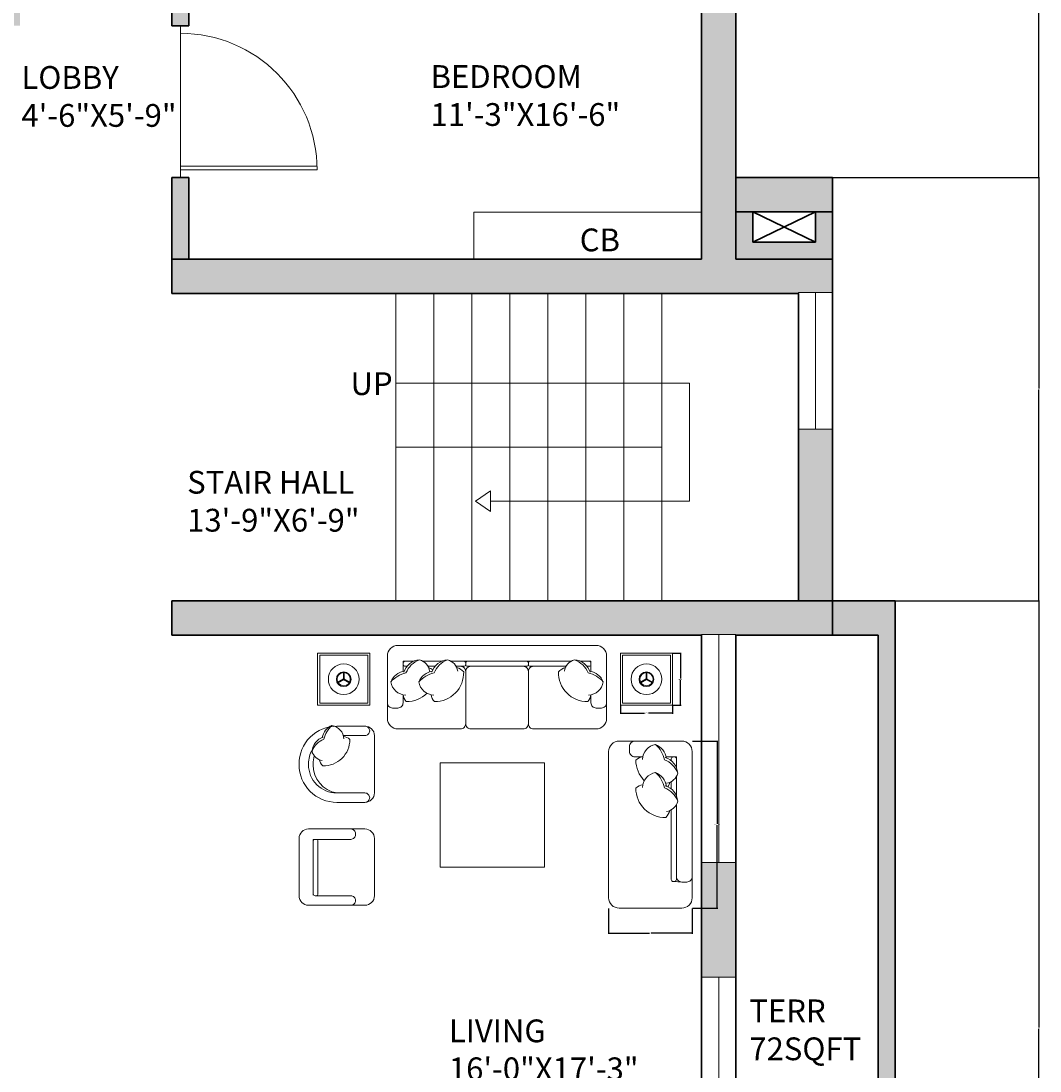
# Model space of a CAD drawing. Units: inches. Extents: x -36 to 442, y -676 to 151.
# Tile 4 of 8: x 174 to 442, y -411 to -134. Entities that reach past the tile are written whole.
import ezdxf

# ---------------------------------------------------------------- set-up
doc = ezdxf.new("R2010")
doc.units = ezdxf.units.IN
doc.header["$MEASUREMENT"] = 0
for name, color, linetype, lineweight in [('A-ANNO-DIMS', 2, 'Continuous', 18), ('A-ANNO-SYMB', 7, 'Continuous', 18), ('A-ANNO-TEXT', 7, 'Continuous', 18), ('A-AREA-IDEN', 7, 'Continuous', 18), ('A-DOOR', 4, 'Continuous', 18), ('A-FLOR-CASE', 32, 'Continuous', 18), ('A-FLOR-STRS', 7, 'Continuous', 18), ('A-FURN', 9, 'Continuous', 13), ('A-GLAZ', 4, 'Continuous', 13), ('A-WALL', 7, 'Continuous', 35), ('A-WALL-PATT', 8, 'Continuous', 13)]:
    doc.layers.add(name, color=color, linetype=linetype, lineweight=lineweight)
doc.styles.get("Standard").update_dxf_attribs({"font": 'arial.ttf'})
doc.dimstyles.get("Standard").update_dxf_attribs({"dimtxt": 0.18, "dimasz": 0.18, "dimexe": 0.18, "dimexo": 0.0625, "dimgap": 0.09, "dimtad": 0, "dimtih": 1, "dimtoh": 1, "dimdec": 0, "dimzin": 0, "dimdsep": 46, "dimlunit": 3, "dimtxsty": 'Standard', "dimcen": 0.09, "dimadec": 0, "dimazin": 0, "dimtfac": 1, "dimtdec": 0, "dimtofl": 0, "dimtmove": 0, "dimatfit": 3, "dimfxl": 1, "dimtolj": 1, "dimtzin": 0, "dimarcsym": 0})

# ---------------------------------------------------------------- blocks, each defined once
blk = doc.blocks.new('DAY BED1')
at = {"color": 0}
blk.add_line((0.3, 0.25), (0.225, 0.255), dxfattribs=at)
blk.add_lwpolyline([(-0.3, 0, -0.414214), (-0.4, 0.1), (-0.4, 0.1, 0.317837), (-0.4, 0.1, -0.414214), (-0.4, 0.1), (-0.4, 0.1, 1.186185), (-0.4, 0.1, -0.414214), (-0.4, 0.1), (-0.4, 1.5, -0.414214), (-0.3, 1.6), (0.3, 1.6, -0.414214), (0.4, 1.5), (0.4, 0.1, -0.414214), (0.3, 0)], format="xyb", close=True, dxfattribs=at)
for points in [[(-0.073, 1.45), (-0.15, 1.45, -0.414214), (-0.2, 1.5), (-0.2, 1.55, -0.414214), (-0.15, 1.6)], [(-0.076, 1.425, -0.356772), (0.05, 1.568, -0.249542), (0.154, 1.438, 9.61688)], [(0.05, 1.568, -0.14773), (0.136, 1.422, -0.213343), (0.262, 1.293, -0.178662)], [(-0.073, 1.45, 0.165541), (-0.139, 1.419, 0.200231), (-0.058, 1.221, 0.121523)], [(0.143, 1.442, -0.306663), (0.262, 1.293, -0.30633), (0.154, 1.196, 0.872847)], [(0.25, 1.345), (0.25, 1.45), (0.152, 1.45, -0.414214)], [(0.2, 1.412), (0.2, 1.43, -0.414214), (0.22, 1.45), (0.23, 1.45, -0.414214), (0.25, 1.43)], [(0.25, 1.43), (0.25, 1.345, -0.414214)], [(-0.076, 1.156, -0.356772), (0.05, 1.299, -0.249542), (0.154, 1.169, 9.61688)], [(0.05, 1.299, -0.14773), (0.136, 1.153, -0.213343), (0.262, 1.024, -0.178662)], [(0.2, 1.142), (0.2, 1.211, -0.414214)], [(0.25, 1.262), (0.25, 1.075, -0.414214)], [(-0.073, 1.181, 0.165541), (-0.139, 1.15, 0.425989), (0.148, 0.869, 0.121523), (0.187, 0.936, -7.115464)], [(0.143, 1.173, -0.306663), (0.262, 1.024, -0.30633), (0.154, 0.926, 0.872847)], [(0.168, 1.163, 0.071865), (0.187, 1.205, -7.115464)], [(0.25, 0.992), (0.25, 0.275, -0.414214), (0.23, 0.255), (0.22, 0.255, -0.414214), (0.2, 0.275), (0.2, 0.942, -0.414214)], [(0.25, 0.377), (0.25, 0.3, 0.414214), (0.3, 0.25), (0.35, 0.25, 0.414214), (0.4, 0.3)]]:
    blk.add_lwpolyline(points, format="xyb", dxfattribs=at)
for points in [[(0.25, 1.075), (0.25, 1.262)], [(0.25, 0.377), (0.25, 0.992)]]:
    blk.add_lwpolyline(points, dxfattribs=at)
blk = doc.blocks.new('END-TABLE-SQUARE')
for p, q in [((6.79, 6.87), (6.79, 8.81)), ((6.96, 6.87), (6.96, 8.81)), ((6.83, 6.95), (5.15, 5.98)), ((6.92, 6.8), (5.24, 5.83)), ((6.83, 6.8), (8.51, 5.83)), ((6.92, 6.95), (8.59, 5.98))]:
    blk.add_line(p, q)
at = {"ltscale": 0.03}
blk.add_lwpolyline([(13.75, 0), (0, 0), (0, 13.75), (13.75, 13.75)], close=True, dxfattribs=at)
blk.add_lwpolyline([(0.55, 0.55), (13.2, 0.55), (13.2, 13.2), (0.55, 13.2)], close=True)
for radius in [4.05, 1.94, 1.74]:
    blk.add_circle((6.87, 6.87), radius)
blk = doc.blocks.new('GLAZING-UNIT-96IN')
for p, q in [((0, 0), (0, 96)), ((4.5, 96), (4.5, 0)), ((9, 96), (9, 0))]:
    blk.add_line(p, q)
blk = doc.blocks.new('*D37')
at = {"layer": 'A-ANNO-DIMS', "color": 0, "lineweight": -2, "transparency": 16777216}
for p, q in [((350.8, -323.93), (357.52, -323.93)), ((357.34, -324.11), (357.34, -345.74)), ((357.34, -367.74), (357.34, -346.1)), ((350.8, -367.92), (357.52, -367.92))]:
    blk.add_line(p, q, dxfattribs=at)
at = {"layer": 'A-ANNO-DIMS', "color": 0, "transparency": 16777216}
for points in [[(357.31, -324.11), (357.37, -324.11), (357.34, -323.93)], [(357.31, -367.74), (357.37, -367.74), (357.34, -367.92)]]:
    blk.add_solid(points, dxfattribs=at)
at = {"layer": 'Defpoints', "color": 0, "transparency": 16777216}
for p in [(350.74, -323.93), (357.34, -323.93), (350.74, -367.92)]:
    blk.add_point(p, dxfattribs=at)
at = {"layer": 'A-ANNO-DIMS', "color": 0, "transparency": 16777216, "insert": (357.34, -345.92), "char_height": 0.18, "attachment_point": 5}
blk.add_mtext('\\A1;DAY BED 44', dxfattribs=at)
blk = doc.blocks.new('*D38')
at = {"layer": 'A-ANNO-DIMS', "color": 0, "lineweight": -2, "transparency": 16777216}
for p, q in [((328.75, -367.98), (328.75, -374.69)), ((350.74, -367.98), (350.74, -374.69)), ((328.93, -374.51), (339.53, -374.51)), ((350.56, -374.51), (339.96, -374.51))]:
    blk.add_line(p, q, dxfattribs=at)
at = {"layer": 'A-ANNO-DIMS', "color": 0, "transparency": 16777216}
for points in [[(328.93, -374.48), (328.93, -374.54), (328.75, -374.51)], [(350.56, -374.48), (350.56, -374.54), (350.74, -374.51)]]:
    blk.add_solid(points, dxfattribs=at)
at = {"layer": 'Defpoints', "color": 0, "transparency": 16777216}
for p in [(328.75, -367.92), (350.74, -367.92), (350.74, -374.51)]:
    blk.add_point(p, dxfattribs=at)
at = {"layer": 'A-ANNO-DIMS', "color": 0, "transparency": 16777216, "insert": (339.74, -374.51), "char_height": 0.18, "attachment_point": 5}
blk.add_mtext('\\A1;22', dxfattribs=at)
blk = doc.blocks.new('*D39')
at = {"layer": 'A-ANNO-DIMS', "color": 0, "lineweight": -2, "transparency": 16777216}
for p, q in [((345.65, -300.75), (347.83, -300.75)), ((347.65, -300.93), (347.65, -307.44)), ((347.65, -314.31), (347.65, -307.8)), ((345.65, -314.49), (347.83, -314.49))]:
    blk.add_line(p, q, dxfattribs=at)
at = {"layer": 'A-ANNO-DIMS', "color": 0, "transparency": 16777216}
for points in [[(347.62, -300.93), (347.68, -300.93), (347.65, -300.75)], [(347.62, -314.31), (347.68, -314.31), (347.65, -314.49)]]:
    blk.add_solid(points, dxfattribs=at)
at = {"layer": 'Defpoints', "color": 0, "transparency": 16777216}
for p in [(345.58, -300.75), (347.65, -300.75), (345.58, -314.49)]:
    blk.add_point(p, dxfattribs=at)
at = {"layer": 'A-ANNO-DIMS', "color": 0, "transparency": 16777216, "insert": (347.65, -307.62), "char_height": 0.18, "attachment_point": 5}
blk.add_mtext('\\A1;TABLE 14 TYP.', dxfattribs=at)
blk = doc.blocks.new('*D40')
at = {"layer": 'A-ANNO-DIMS', "color": 0, "lineweight": -2, "transparency": 16777216}
for p, q in [((331.84, -314.56), (331.84, -316.74)), ((345.58, -314.56), (345.58, -316.74)), ((332.02, -316.56), (338.19, -316.56)), ((345.4, -316.56), (339.23, -316.56))]:
    blk.add_line(p, q, dxfattribs=at)
at = {"layer": 'A-ANNO-DIMS', "color": 0, "transparency": 16777216}
for points in [[(332.02, -316.53), (332.02, -316.59), (331.84, -316.56)], [(345.4, -316.53), (345.4, -316.59), (345.58, -316.56)]]:
    blk.add_solid(points, dxfattribs=at)
at = {"layer": 'Defpoints', "color": 0, "transparency": 16777216}
for p in [(331.84, -314.49), (345.58, -314.49), (345.58, -316.56)]:
    blk.add_point(p, dxfattribs=at)
at = {"layer": 'A-ANNO-DIMS', "color": 0, "transparency": 16777216, "insert": (338.71, -316.56), "char_height": 0.18, "attachment_point": 5}
blk.add_mtext('\\A1;14 TYP.', dxfattribs=at)
blk = doc.blocks.new('*D49')
at = {"layer": 'A-ANNO-DIMS', "color": 0, "lineweight": -2, "transparency": 16777216}
for p, q in [((2.24, -363.56), (2.24, -675.98)), ((404.24, -512.06), (404.24, -675.98)), ((2.42, -675.8), (202.94, -675.8)), ((404.06, -675.8), (203.53, -675.8))]:
    blk.add_line(p, q, dxfattribs=at)
at = {"layer": 'A-ANNO-DIMS', "color": 0, "transparency": 16777216}
for points in [[(2.42, -675.77), (2.42, -675.83), (2.24, -675.8)], [(404.06, -675.77), (404.06, -675.83), (404.24, -675.8)]]:
    blk.add_solid(points, dxfattribs=at)
at = {"layer": 'Defpoints', "color": 0, "transparency": 16777216}
for p in [(2.24, -363.5), (404.24, -512), (404.24, -675.8)]:
    blk.add_point(p, dxfattribs=at)
at = {"layer": 'A-ANNO-DIMS', "color": 0, "transparency": 16777216, "insert": (203.24, -675.8), "char_height": 0.18, "attachment_point": 5}
blk.add_mtext('\\A1;402', dxfattribs=at)
blk = doc.blocks.new('*D57')
at = {"layer": 'A-ANNO-DIMS', "color": 0, "lineweight": -2, "transparency": 16777216}
for p, q in [((378.8, 1), (442.22, 1)), ((442.04, 0.82), (442.04, -87.07)), ((442.04, -175.32), (442.04, -87.43)), ((387.8, -175.5), (442.22, -175.5))]:
    blk.add_line(p, q, dxfattribs=at)
at = {"layer": 'A-ANNO-DIMS', "color": 0, "transparency": 16777216}
for points in [[(442.01, 0.82), (442.07, 0.82), (442.04, 1)], [(442.01, -175.32), (442.07, -175.32), (442.04, -175.5)]]:
    blk.add_solid(points, dxfattribs=at)
at = {"layer": 'Defpoints', "color": 0, "transparency": 16777216}
for p in [(378.74, 1), (387.74, -175.5), (442.04, -175.5)]:
    blk.add_point(p, dxfattribs=at)
at = {"layer": 'A-ANNO-DIMS', "color": 0, "transparency": 16777216, "insert": (442.04, -87.25), "char_height": 0.18, "attachment_point": 5}
blk.add_mtext('\\A1;176.5', dxfattribs=at)
blk = doc.blocks.new('*D58')
at = {"layer": 'A-ANNO-DIMS', "color": 0, "lineweight": -2, "transparency": 16777216}
for p, q in [((387.8, -175.5), (442.22, -175.5)), ((442.04, -175.68), (442.04, -231.07)), ((442.04, -286.82), (442.04, -231.43)), ((404.3, -287), (442.22, -287))]:
    blk.add_line(p, q, dxfattribs=at)
at = {"layer": 'A-ANNO-DIMS', "color": 0, "transparency": 16777216}
for points in [[(442.01, -175.68), (442.07, -175.68), (442.04, -175.5)], [(442.01, -286.82), (442.07, -286.82), (442.04, -287)]]:
    blk.add_solid(points, dxfattribs=at)
at = {"layer": 'Defpoints', "color": 0, "transparency": 16777216}
for p in [(387.74, -175.5), (404.24, -287), (442.04, -287)]:
    blk.add_point(p, dxfattribs=at)
at = {"layer": 'A-ANNO-DIMS', "color": 0, "transparency": 16777216, "insert": (442.04, -231.25), "char_height": 0.18, "attachment_point": 5}
blk.add_mtext('\\A1;111.5', dxfattribs=at)
blk = doc.blocks.new('*D59')
at = {"layer": 'A-ANNO-DIMS', "color": 0, "lineweight": -2, "transparency": 16777216}
for p, q in [((404.3, -287), (442.22, -287)), ((442.04, -287.18), (442.04, -399.32)), ((442.04, -511.82), (442.04, -399.68)), ((404.3, -512), (442.22, -512))]:
    blk.add_line(p, q, dxfattribs=at)
at = {"layer": 'A-ANNO-DIMS', "color": 0, "transparency": 16777216}
for points in [[(442.01, -287.18), (442.07, -287.18), (442.04, -287)], [(442.01, -511.82), (442.07, -511.82), (442.04, -512)]]:
    blk.add_solid(points, dxfattribs=at)
at = {"layer": 'Defpoints', "color": 0, "transparency": 16777216}
for p in [(404.24, -287), (404.24, -512), (442.04, -512)]:
    blk.add_point(p, dxfattribs=at)
at = {"layer": 'A-ANNO-DIMS', "color": 0, "transparency": 16777216, "insert": (442.04, -399.5), "char_height": 0.18, "attachment_point": 5}
blk.add_mtext('\\A1;225', dxfattribs=at)

msp = doc.modelspace()

# ---------------------------------------------------------------- hatches: boundary and pattern name
at = {"layer": 'A-WALL-PATT'}
h = msp.add_hatch(color=256, dxfattribs=at)
h.dxf.hatch_style = 1
h.paths.add_polyline_path([(288, 113.503), (193.5, 113.503), (97.5, 113.503), (97.5, 104.864), (106.5, 104.864), (106.5, 104.503), (193.5, 104.503), (193.5, 5.503), (193.5, 1.003), (213.735, 1.003), (213.735, -135.497), (218.235, -135.497), (218.235, 1.003), (251, 1.003), (251, 3.253), (251, 5.503), (198, 5.503), (198, 104.503), (279, 104.503), (279, 104.209), (288, 104.209)])
h.paths.add_polyline_path([(378.735, 81.646), (362.235, 81.646), (288, 81.646), (288, 80.209), (279, 80.209), (279, 5.503), (279, 1.003), (353.235, 1.003), (353.235, 0.242), (362.235, 0.242), (362.235, 5.503), (288, 5.503), (288, 77.146), (362.235, 77.146), (374.235, 77.146), (374.235, 5.503), (362.235, 5.503), (362.235, 1.003), (374.235, 1.003), (378.735, 1.003), (378.735, 5.503), (378.735, 77.146)])
h.paths.add_polyline_path([(362.235, -35.758), (353.235, -35.758), (353.235, -196.997), (218.235, -196.997), (213.735, -196.997), (213.735, -205.997), (218.235, -205.997), (378.735, -205.997), (378.735, -205.779), (387.735, -205.779), (387.735, -202.472), (387.735, -196.997), (378.735, -196.997), (362.235, -196.997)])
h.paths.add_polyline_path([(218.235, -175.497), (215.985, -175.497), (213.735, -175.497), (213.735, -196.997), (218.235, -196.997)], flags=17)
h.paths.add_polyline_path([(158.235, -201.497), (98.235, -201.497), (98.235, -205.997), (158.235, -205.997)])
h.paths.add_polyline_path([(173.735, -130.997), (27.735, -130.997), (27.735, -35.267), (18.735, -35.267), (18.735, -138.68), (27.735, -138.68), (27.735, -135.497), (93.735, -135.497), (93.735, -201.497), (98.235, -201.497), (98.235, -135.497), (158.235, -135.497), (158.235, -173.497), (160.739, -173.497), (162.735, -173.497), (162.735, -135.497), (173.735, -135.497), (173.735, -133.017)])
h.paths.add_polyline_path([(98.235, -201.497), (93.735, -201.497), (93.735, -205.997), (98.235, -205.997)])
h.paths.add_polyline_path([(162.735, -201.497), (158.235, -201.497), (158.235, -205.997), (162.735, -205.997)])
h.paths.add_polyline_path([(63.735, -205.997), (63.735, -201.497), (27.735, -201.497), (27.735, -162.68), (18.735, -162.68), (18.735, -210.497), (63.735, -210.497)])
h.paths.add_polyline_path([(65.735, -203.604), (65.735, -201.497), (63.735, -201.497), (63.735, -205.997), (65.735, -205.997)])
h.paths.add_polyline_path([(165.5, 5.503), (106.5, 5.503), (106.5, 80.864), (97.5, 80.864), (97.5, 81.646), (6.735, 81.646), (2.235, 81.646), (2.235, 77.146), (2.235, 5.503), (2.235, 1.003), (6.735, 1.003), (18.735, 1.003), (18.735, 5.503), (6.735, 5.503), (6.735, 77.146), (97.5, 77.146), (97.5, 5.503), (18.735, 5.503), (18.735, 0.733), (27.735, 0.733), (27.735, 1.003), (165.5, 1.003), (165.5, 3.253)])
h.paths.add_polyline_path([(18.735, -201.497), (6.735, -201.497), (2.235, -201.497), (2.235, -210.497), (2.235, -354.497), (2.235, -363.497), (6.735, -363.497), (18.735, -363.497), (18.735, -358.997), (18.735, -354.497), (6.735, -354.497), (6.735, -210.497), (18.735, -210.497)])
h.paths.add_polyline_path([(63.735, -210.497), (54.735, -210.497), (54.735, -240.747), (63.735, -240.747)])
h.paths.add_polyline_path([(63.735, -336.747), (54.735, -336.747), (54.735, -354.497), (18.735, -354.497), (18.735, -358.997), (18.735, -363.497), (104.735, -363.497), (104.735, -361.247), (104.735, -358.997), (63.735, -358.997)])
h.paths.add_polyline_path([(27.735, -448.151), (18.735, -448.151), (18.735, -637.997), (72.735, -637.997), (72.735, -571.997), (183.235, -571.997), (183.235, -562.997), (57.197, -562.997), (51.735, -562.997), (51.735, -567.497), (57.197, -567.497), (63.735, -567.497), (63.735, -571.997), (63.735, -628.997), (27.735, -628.997), (27.735, -475.997), (27.735, -471.497)])
h.paths.add_polyline_path([(27.735, -363.497), (18.735, -363.497), (18.735, -412.151), (27.735, -412.151)])
h.paths.add_polyline_path([(161.235, -358.997), (132.735, -358.997), (132.735, -363.497), (156.735, -363.497), (156.735, -471.497), (51.735, -471.497), (51.735, -475.997), (63.735, -475.997), (63.735, -534.997), (65.985, -534.997), (68.235, -534.997), (68.235, -475.997), (161.235, -475.997)])
h.paths.add_polyline_path([(161.235, -511.997), (173.235, -511.997), (173.235, -502.997), (161.235, -502.997), (161.235, -475.997), (152.235, -475.997), (152.235, -534.997), (156.735, -534.997), (161.235, -534.997)], flags=17)
h.paths.add_polyline_path([(362.235, -502.997), (353.235, -502.997), (213.235, -502.997), (213.235, -507.497), (213.235, -511.997), (362.235, -511.997)])
h.paths.add_polyline_path([(242.235, -548.019), (233.235, -548.019), (233.235, -562.997), (223.235, -562.997), (223.235, -567.497), (223.235, -571.997), (242.235, -571.997)])
h.paths.add_polyline_path([(404.235, -502.997), (399.735, -502.997), (362.235, -502.997), (362.235, -511.997), (399.735, -511.997), (404.235, -511.997)])
h.paths.add_polyline_path([(362.235, -482.123), (353.235, -482.123), (353.235, -502.997), (362.235, -502.997)])
h.paths.add_polyline_path([(404.235, -295.997), (404.235, -286.997), (387.735, -286.997), (387.735, -295.997), (399.735, -295.997), (399.735, -502.997), (404.235, -502.997)])
h.paths.add_polyline_path([(362.235, -355.863), (353.235, -355.863), (353.235, -386.123), (362.235, -386.123)])
h.paths.add_polyline_path([(387.735, -286.997), (378.735, -286.997), (213.735, -286.997), (213.735, -295.997), (353.235, -295.997), (353.235, -295.863), (362.235, -295.863), (362.235, -295.997), (378.735, -295.997), (387.735, -295.997)])
h.paths.add_polyline_path([(387.735, -241.779), (378.735, -241.779), (378.735, -286.997), (387.735, -286.997)])
h.paths.add_polyline_path([(387.735, -175.497), (362.235, -175.497), (362.235, -184.497), (387.735, -184.497)], flags=17)
h.paths.add_polyline_path([(387.735, -184.497), (383.235, -184.497), (383.235, -192.497), (378.735, -192.497), (366.735, -192.497), (366.735, -184.497), (362.235, -184.497), (362.235, -196.997), (378.735, -196.997), (387.735, -196.997)], flags=17)
h.paths.add_polyline_path([(240.604, 40.967), (282.575, 40.967), (282.575, 63.356), (240.604, 63.356)], flags=25)

# ---------------------------------------------------------------- linework, layer by layer
at = {"layer": 'A-ANNO-SYMB'}
for p, q in [((272.735, -229.643), (350.047, -229.643)), ((350.047, -229.643), (350.047, -260.735)), ((297.61, -258.047), (293.659, -260.735)), ((297.61, -260.735), (297.61, -258.047)), ((297.61, -263.424), (293.659, -260.735)), ((350.047, -260.735), (297.61, -260.735)), ((297.61, -260.735), (297.61, -263.424))]:
    msp.add_line(p, q, dxfattribs=at)
at = {"layer": 'A-DOOR'}
for p, q in [((215.985, -135.497), (215.985, -137.497)), ((215.985, -173.497), (215.985, -137.497)), ((215.985, -172.497), (251.985, -172.497)), ((215.985, -173.497), (215.985, -175.497)), ((215.985, -173.497), (251.985, -173.497))]:
    msp.add_line(p, q, dxfattribs=at)
msp.add_arc((215.985, -173.497), 36, 0, 90, dxfattribs=at)
at = {"layer": 'A-FLOR-CASE'}
for p, q in [((353.235, -184.643), (293.235, -184.643)), ((293.235, -184.643), (293.235, -196.997))]:
    msp.add_line(p, q, dxfattribs=at)
at = {"layer": 'A-FLOR-STRS'}
for p, q in [((272.735, -205.997), (272.735, -286.997)), ((282.735, -205.997), (282.735, -286.997)), ((292.735, -205.997), (292.735, -286.997)), ((302.735, -205.997), (302.735, -286.997)), ((312.735, -205.997), (312.735, -286.997)), ((322.735, -205.997), (322.735, -286.997)), ((332.735, -205.997), (332.735, -286.997)), ((342.735, -205.997), (342.735, -286.997)), ((342.735, -246.497), (272.735, -246.497))]:
    msp.add_line(p, q, dxfattribs=at)
at = {"layer": 'A-FURN', "ltscale": 0.03}
for points in [[(328.227, -317.969, -0.4142136), (325.478, -320.718), (308.984, -320.718, -0.4142136), (307.61, -319.343, -0.4142136), (306.235, -320.718), (292.49, -320.718, -0.4142136), (291.116, -319.343, -0.4142136), (289.741, -320.718), (273.247, -320.718, -0.4142136), (270.498, -317.969), (270.498, -301.475, -0.4142136), (273.247, -298.726), (325.478, -298.726, -0.4142136), (328.227, -301.475)], [(247.241, -364.67), (247.241, -364.67, 0.4142136), (249.72, -367.149), (264.591, -367.149, 0.4142136), (267.07, -364.67), (267.07, -364.67), (267.07, -349.551, 0.4142136), (264.591, -347.072), (249.72, -347.072, 0.4142136), (247.241, -349.551)]]:
    msp.add_lwpolyline(points, format="xyb", close=True, dxfattribs=at)
at = {"layer": 'A-FURN'}
for points in [[(271.373, -308.334, -0.1477299), (275.39, -305.972, -0.2133428), (278.935, -302.507, -0.1786618)], [(277.513, -302.849), (274.622, -302.849), (274.622, -305.55, -0.4142136)], [(275.671, -304.224), (275.171, -304.224, -0.4142136), (274.622, -303.674), (274.622, -303.399, -0.4142136), (275.171, -302.849)], [(274.835, -305.784, -0.3066635), (278.935, -302.507, -0.30633), (281.613, -305.5, 0.8728472)], [(275.171, -302.849), (277.513, -302.849, -0.4142136)], [(278.777, -308.334, -0.1477299), (282.795, -305.972, -0.2133428), (286.339, -302.507, -0.1786618)], [(279.8, -302.849), (284.918, -302.849, -0.4142136)], [(282.24, -305.784, -0.3066635), (286.339, -302.507, -0.30633), (289.017, -305.5, 0.8728472)], [(287.204, -302.849), (290.566, -302.849, -0.4142136), (291.116, -303.399), (291.116, -303.674, -0.4142136), (290.566, -304.224), (288.588, -304.224, -0.4142136)], [(318.926, -302.849), (308.16, -302.849, 0.4142136), (307.61, -303.399), (307.61, -303.674, 0.4142136), (308.16, -304.224), (317.542, -304.224, 0.4142136)], [(323.89, -305.784, 0.3066635), (319.791, -302.507, 0.30633), (317.112, -305.5, -0.8728472)], [(327.353, -308.334, 0.1477299), (323.335, -305.972, 0.2133428), (319.791, -302.507, 0.1786618)], [(323.554, -302.849), (321.212, -302.849, 0.4142136)], [(323.055, -304.224), (323.554, -304.224, 0.4142136), (324.104, -303.674), (324.104, -303.399, 0.4142136), (323.554, -302.849)], [(275.311, -311.799, -0.3567724), (271.373, -308.334, -0.2495421), (274.942, -305.479, 9.6168803)], [(282.716, -311.799, -0.3567724), (278.777, -308.334, -0.2495421), (282.346, -305.479, 9.6168803)], [(283.075, -304.224), (281.184, -304.224, -0.4142136)], [(282.508, -305.109, 0.0718654), (281.356, -304.572, -7.1154643)], [(282.023, -311.715, 0.1655406), (282.873, -313.531, 0.4259892), (290.593, -305.657, 0.1215233), (288.76, -304.572, -7.1154643)], [(289.741, -304.224, -0.4142136), (291.116, -305.598), (291.116, -319.343, -0.4142136)], [(292.49, -304.224, 0.4142136), (291.116, -305.598)], [(306.235, -304.224, -0.4142136), (307.61, -305.598)], [(308.984, -304.224, 0.4142136), (307.61, -305.598), (307.61, -319.343, 0.4142136)], [(324.107, -311.715, -0.1655406), (323.257, -313.531, -0.4259892), (315.537, -305.657, -0.1215233), (317.369, -304.572, 7.1154643)], [(323.414, -311.799, 0.3567724), (327.353, -308.334, 0.2495421), (323.784, -305.479, -9.6168803)], [(274.622, -311.716), (274.622, -313.845, -0.4142136), (273.247, -315.22), (271.873, -315.22, -0.4142136), (270.498, -313.845)], [(274.619, -311.715, 0.1655406), (275.469, -313.531, 0.2002311), (280.925, -311.319, 0.1215233)], [(328.227, -313.845, -0.4142136), (326.853, -315.22), (325.478, -315.22, -0.4142136), (324.104, -313.845), (324.104, -311.716)], [(255.904, -319.786, 0.1477299), (253.775, -323.408, 0.2133428), (250.651, -326.604, 0.1786618)], [(259.028, -323.337, 0.3567724), (255.904, -319.786, 0.2495421), (253.33, -323.003, -9.6168803)], [(258.893, -322.467), (264.591, -322.467, 0.4142136), (265.831, -321.228), (265.831, -321.228, 0.4142136), (264.591, -319.988)], [(253.605, -322.907, 0.3066635), (250.651, -326.604, 0.30633), (253.349, -329.019, -0.8728472)], [(258.953, -322.712, -0.1655406), (260.59, -323.479, -0.4259892), (253.491, -330.439, -0.1215233), (252.512, -328.787, 7.1154643)], [(250.7, -326.212, 0.1305915), (249.72, -329.903), (249.72, -330.027)], [(251.226, -327.79, 0.0723842), (250.959, -329.903), (250.959, -330.027)], [(257.155, -337.586, -0.4142136), (249.72, -330.151), (249.72, -330.027)], [(257.155, -337.586, -0.3727189), (250.959, -330.151), (250.959, -330.027)], [(257.155, -337.586), (264.591, -337.586, -0.4142136), (265.831, -338.826), (265.831, -338.826, -0.4142136), (264.591, -340.065)], [(260.873, -347.072, -0.4142136), (262.113, -348.311), (262.113, -348.559, -0.4142136), (260.873, -349.799), (258.953, -349.799)], [(252.198, -355.715), (252.198, -350.294, 0.4142136), (251.703, -349.799), (251.455, -349.799, 0.4142136), (250.959, -350.294)], [(250.959, -350.294), (250.959, -354.467, 0.4142136)], [(250.959, -354.467), (250.959, -364.175, 0.4142136), (251.455, -364.67), (251.703, -364.67, 0.4142136), (252.198, -364.175), (252.198, -355.715, 0.4142136)], [(251.703, -364.67), (260.873, -364.67, -0.4142136), (262.113, -365.91), (262.113, -365.91, -0.4142136), (260.873, -367.149)]]:
    msp.add_lwpolyline(points, format="xyb", dxfattribs=at)
for points in [[(284.918, -302.849), (279.8, -302.849)], [(318.926, -302.849), (287.204, -302.849)], [(324.104, -305.55), (324.104, -302.849), (321.212, -302.849)], [(258.953, -349.799), (250.959, -349.799), (250.959, -354.467)], [(250.959, -354.467), (250.959, -364.546)]]:
    msp.add_lwpolyline(points, dxfattribs=at)
msp.add_lwpolyline([(291.665, -302.849), (307.06, -302.849, -0.4142136), (307.61, -303.399), (307.61, -303.674, -0.4142136), (307.06, -304.224), (291.665, -304.224, -0.4142136), (291.116, -303.674), (291.116, -303.399, -0.4142136)], format="xyb", close=True, dxfattribs=at)
at = {"layer": 'A-FURN', "ltscale": 0.03}
msp.add_lwpolyline([(267.07, -330.027), (267.07, -337.586, -0.4142136), (264.591, -340.065), (257.155, -340.065, -0.4142136), (247.241, -330.151), (247.241, -330.027), (247.241, -329.903, -0.4142136), (257.155, -319.988), (264.591, -319.988, -0.4142136), (267.07, -322.467), (267.07, -330.027)], format="xyb", dxfattribs=at)
msp.add_lwpolyline([(284.418, -357.104), (311.908, -357.104), (311.908, -329.614), (284.418, -329.614)], close=True, dxfattribs=at)
at = {"layer": 'A-GLAZ'}
for p, q in [((378.735, -205.779), (378.735, -241.779)), ((387.735, -205.779), (378.735, -205.779)), ((383.235, -205.779), (383.235, -241.779)), ((387.735, -241.779), (387.735, -205.779)), ((378.735, -241.779), (387.735, -241.779)), ((353.235, -355.863), (353.235, -295.863)), ((353.235, -295.863), (362.235, -295.863)), ((357.735, -295.863), (357.735, -355.863)), ((362.235, -295.863), (362.235, -355.863)), ((362.235, -355.863), (353.235, -355.863)), ((353.235, -386.123), (362.235, -386.123))]:
    msp.add_line(p, q, dxfattribs=at)
at = {"layer": 'A-WALL'}
for p, q in [((362.235, 5.503), (362.235, -196.997)), ((213.735, 1.003), (213.735, -135.497)), ((218.235, 1.003), (218.235, -135.497)), ((353.235, 1.003), (353.235, -196.997)), ((213.735, -135.497), (218.235, -135.497)), ((215.985, -175.497), (213.735, -175.497)), ((213.735, -175.497), (213.735, -205.997)), ((215.985, -175.497), (218.235, -175.497)), ((218.235, -175.497), (218.235, -196.997)), ((362.235, -175.497), (387.735, -175.497)), ((387.735, -175.497), (387.735, -196.997)), ((362.235, -184.497), (387.735, -184.497)), ((366.735, -184.497), (366.735, -192.497)), ((366.735, -184.497), (383.235, -192.497)), ((383.235, -184.497), (366.735, -192.497)), ((383.235, -184.497), (383.235, -192.497)), ((366.735, -192.497), (378.735, -192.497)), ((378.735, -192.497), (383.235, -192.497)), ((213.735, -196.997), (218.235, -196.997)), ((218.235, -196.997), (353.235, -196.997)), ((362.235, -196.997), (378.735, -196.997)), ((378.735, -196.997), (387.735, -196.997)), ((387.735, -196.997), (387.735, -202.472)), ((387.735, -202.472), (387.735, -205.997)), ((213.735, -205.997), (378.735, -205.997)), ((213.735, -205.997), (218.235, -205.997)), ((378.735, -205.997), (378.735, -286.997)), ((387.735, -205.997), (387.735, -286.997)), ((213.735, -286.997), (378.735, -286.997)), ((213.735, -286.997), (213.735, -295.997)), ((378.735, -286.997), (404.235, -286.997)), ((387.735, -295.997), (387.735, -286.997)), ((404.235, -286.997), (404.235, -295.997)), ((213.735, -295.997), (353.235, -295.997)), ((353.235, -295.997), (353.235, -502.997)), ((362.235, -295.997), (362.235, -511.997)), ((362.235, -295.997), (378.735, -295.997)), ((378.735, -295.997), (387.735, -295.997)), ((387.735, -295.997), (399.735, -295.997)), ((399.735, -295.997), (399.735, -502.997)), ((404.235, -295.997), (404.235, -502.997))]:
    msp.add_line(p, q, dxfattribs=at)

# ---------------------------------------------------------------- block references
at = {"layer": 'A-FURN', "extrusion": (0, 0, -1), "zscale": -1}
msp.add_blockref('END-TABLE-SQUARE', (-265.863, -314.495), dxfattribs=at)
at = {"layer": 'A-FURN'}
msp.add_blockref('END-TABLE-SQUARE', (331.838, -314.495), dxfattribs=at)
at = {"layer": 'A-FURN', "ltscale": 0.03, "xscale": 27.49012340210402, "yscale": 27.49012340210402, "zscale": 27.49012340210402}
msp.add_blockref('DAY BED1', (339.745, -367.916), dxfattribs=at)
at = {"layer": 'A-GLAZ'}
msp.add_blockref('GLAZING-UNIT-96IN', (353.235, -482.123), dxfattribs=at)

# ---------------------------------------------------------------- texts
at = {"layer": 'A-ANNO-TEXT', "insert": (321.139, -188.918), "char_height": 6, "attachment_point": 1}
msp.add_mtext_dynamic_manual_height_columns('CB', width=0.45758, gutter_width=1, heights=[0], dxfattribs=at)
at = {"layer": 'A-ANNO-TEXT', "insert": (260.78, -226.771), "char_height": 6, "attachment_point": 1}
msp.add_mtext('UP', dxfattribs=at)
at = {"layer": 'A-AREA-IDEN', "char_height": 6, "attachment_point": 1}
for s, insert in [('LOBBY\\P4\'-6"X5\'-9"', (174.13, -146.129)), ('BEDROOM\\P11\'-3"X16\'-6"', (281.87, -145.889)), ('STAIR HALL\\P13\'-9"X6\'-9"', (217.768, -252.748)), ('TERR\\P72SQFT', (365.801, -391.976)), ('LIVING\\P16\'-0"X17\'-3"', (286.694, -397.246))]:
    msp.add_mtext(s, dxfattribs=dict(at, insert=insert))

# ---------------------------------------------------------------- dimensions: what is measured, and where the dimension line sits
at = {"layer": 'A-ANNO-DIMS'}
for base, p1, p2, override, picture, middle in [((442.035, -175.497), (378.735, 1.003), (387.735, -175.497), {"dimdec": 1, "dimlfac": 1, "dimrnd": 0, "dimzin": 0, "dimdsep": 46, "dimlunit": 2}, '*D57', (442.035, -87.247)), ((442.035, -286.997), (387.735, -175.497), (404.235, -286.997), {"dimdec": 1, "dimlfac": 1, "dimrnd": 0, "dimzin": 0, "dimdsep": 46, "dimlunit": 2}, '*D58', (442.035, -231.247)), ((442.035, -511.997), (404.235, -286.997), (404.235, -511.997), {"dimdec": 0, "dimlfac": 1, "dimrnd": 0, "dimzin": 0, "dimdsep": 46, "dimlunit": 2}, '*D59', (442.035, -399.497))]:
    dim = msp.add_linear_dim(base=base, p1=p1, p2=p2, angle=90, dimstyle='Standard', override=override, dxfattribs=at)
    dim.commit()
    dim.dimension.update_dxf_attribs({"geometry": picture, "text_midpoint": middle})
for base, p1, p2, text, picture, middle in [((347.645, -300.75), (345.583, -314.495), (345.583, -300.75), 'TABLE <> TYP.', '*D39', (347.645, -307.622)), ((357.338, -323.932), (350.741, -367.916), (350.741, -323.932), 'DAY BED <>', '*D37', (357.338, -345.924))]:
    dim = msp.add_linear_dim(base=base, p1=p1, p2=p2, angle=90, text=text, dimstyle='Standard', override={"dimdec": 0, "dimlfac": 1, "dimrnd": 0, "dimzin": 0, "dimdsep": 46, "dimlunit": 2}, dxfattribs=at)
    dim.commit()
    dim.dimension.update_dxf_attribs({"geometry": picture, "text_midpoint": middle})
dim = msp.add_linear_dim(base=(345.583, -316.557), p1=(331.838, -314.495), p2=(345.583, -314.495), text='<> TYP.', dimstyle='Standard', override={"dimdec": 0, "dimlfac": 1, "dimrnd": 0, "dimzin": 0, "dimdsep": 46, "dimlunit": 2}, dxfattribs=at)
dim.commit()
dim.dimension.update_dxf_attribs({"geometry": '*D40', "text_midpoint": (338.711, -316.557)})
for base, p1, p2, picture, middle in [((404.235, -675.797), (2.235, -363.497), (404.235, -511.997), '*D49', (203.235, -675.797)), ((350.741, -374.514), (328.749, -367.916), (350.741, -367.916), '*D38', (339.745, -374.514))]:
    dim = msp.add_linear_dim(base=base, p1=p1, p2=p2, dimstyle='Standard', override={"dimdec": 0, "dimlfac": 1, "dimrnd": 0, "dimzin": 0, "dimdsep": 46, "dimlunit": 2}, dxfattribs=at)
    dim.commit()
    dim.dimension.update_dxf_attribs({"geometry": picture, "text_midpoint": middle})

doc.saveas('drawing.dxf')
